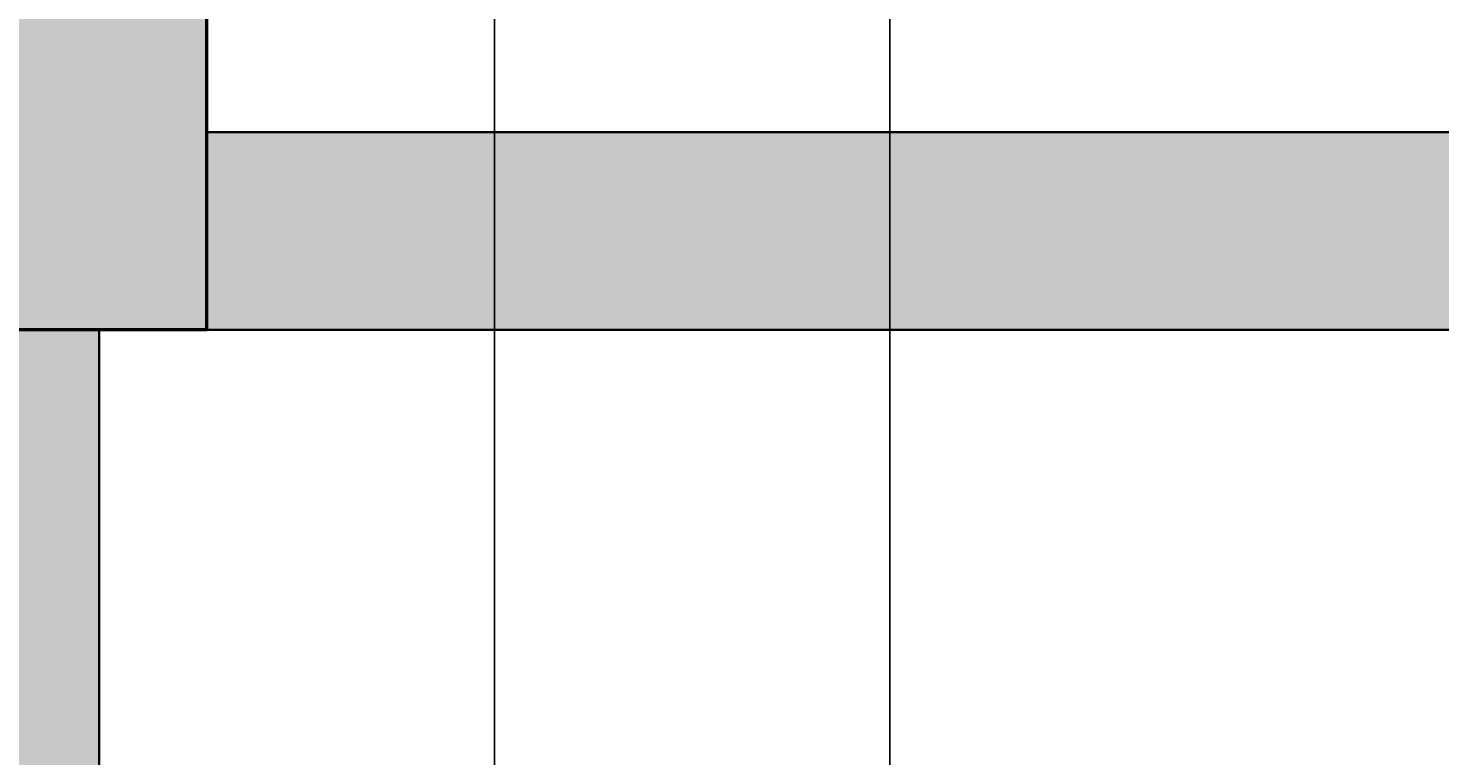
# Model space of a CAD drawing. Units: inches. Extents: x 1998 to 2588, y 1139 to 1977.
# Tile 61 of 134: x 2095 to 2127, y 1746 to 1762. Entities that reach past the tile are written whole.
import ezdxf

# ---------------------------------------------------------------- set-up
doc = ezdxf.new("R2010")
doc.units = ezdxf.units.IN
for name, color, linetype, lineweight in [('A-ANNO-DIMS', 2, 'Continuous', 18), ('A-COLS-PATT', 250, 'Continuous', 13), ('A-WALL-PATT', 252, 'Continuous', 13), ('COLUMN', 10, 'Continuous', 50), ('WALL', 200, 'Continuous', 35)]:
    doc.layers.add(name, color=color, linetype=linetype, lineweight=lineweight)
doc.styles.get("Standard").update_dxf_attribs({"font": 'arial.ttf'})
doc.dimstyles.get("Standard").update_dxf_attribs({"dimtxt": 0.18, "dimasz": 0.18, "dimexe": 0.18, "dimexo": 0.0625, "dimgap": 0.09, "dimtad": 0, "dimtih": 1, "dimtoh": 1, "dimdec": 4, "dimzin": 0, "dimdsep": 46, "dimtxsty": 'Standard', "dimcen": 0.09, "dimadec": 0, "dimazin": 0, "dimtfac": 1, "dimtdec": 4, "dimtofl": 0, "dimtmove": 0, "dimatfit": 3, "dimfxl": 1, "dimtolj": 1, "dimtzin": 0, "dimarcsym": 0})

# ---------------------------------------------------------------- blocks, each defined once
blk = doc.blocks.new('*D40')
at = {"layer": 'A-ANNO-DIMS', "color": 0, "lineweight": -2, "transparency": 16777216}
for p, q in [((2105.973, 1628.541), (2105.973, 1977.362)), ((2114.973, 1628.804), (2114.973, 1977.362)), ((2106.153, 1977.182), (2110.324, 1977.182)), ((2114.793, 1977.182), (2110.622, 1977.182))]:
    blk.add_line(p, q, dxfattribs=at)
at = {"layer": 'A-ANNO-DIMS', "color": 0, "transparency": 16777216}
for points in [[(2106.153, 1977.212), (2106.153, 1977.152), (2105.973, 1977.182)], [(2114.793, 1977.212), (2114.793, 1977.152), (2114.973, 1977.182)]]:
    blk.add_solid(points, dxfattribs=at)
at = {"layer": 'Defpoints', "color": 0, "transparency": 16777216}
for p in [(2114.973, 1977.182), (2114.973, 1628.742), (2105.973, 1628.478)]:
    blk.add_point(p, dxfattribs=at)
at = {"layer": 'A-ANNO-DIMS', "color": 0, "transparency": 16777216, "insert": (2110.473, 1977.182), "char_height": 0.18, "attachment_point": 5}
blk.add_mtext('\\A1;9', dxfattribs=at)

msp = doc.modelspace()

# ---------------------------------------------------------------- hatches: boundary and pattern name
at = {"layer": 'A-COLS-PATT'}
h = msp.add_hatch(color=256, dxfattribs=at)
h.dxf.hatch_style = 1
h.paths.add_polyline_path([(2099.4125, 1888.7324), (2087.9729, 1888.7324), (2087.9729, 1868.3278), (2099.4125, 1868.3278)])
h.paths.add_polyline_path([(2234.4125, 1888.7324), (2222.9729, 1888.7324), (2222.9729, 1868.3278), (2234.4125, 1868.3278)])
h.paths.add_polyline_path([(2341.4729, 1886.637), (2330.0332, 1886.637), (2330.0332, 1866.2324), (2341.4729, 1866.2324)])
h.paths.add_polyline_path([(2507.8006, 1882.7324), (2487.396, 1882.7324), (2487.396, 1871.2927), (2507.8006, 1871.2927)])
h.paths.add_polyline_path([(2510.9729, 1766.672), (2490.5682, 1766.672), (2490.5682, 1755.2324), (2510.9729, 1755.2324)])
h.paths.add_polyline_path([(2345.9729, 1759.7324), (2334.5332, 1759.7324), (2334.5332, 1739.3278), (2345.9729, 1739.3278)])
h.paths.add_polyline_path([(2234.4125, 1774.3318), (2222.9729, 1774.3318), (2222.9729, 1753.9272), (2234.4125, 1753.9272)])
h.paths.add_polyline_path([(2099.4125, 1775.637), (2087.9729, 1775.637), (2087.9729, 1755.2324), (2099.4125, 1755.2324)])
h.paths.add_polyline_path([(2098.0956, 1593.7241), (2077.691, 1593.7241), (2077.691, 1582.2845), (2098.0956, 1582.2845)])
h.paths.add_polyline_path([(2227.4729, 1604.637), (2216.0332, 1604.637), (2216.0332, 1584.2324), (2227.4729, 1584.2324)])
h.paths.add_polyline_path([(2345.9729, 1647.5211), (2334.5332, 1647.5211), (2334.5332, 1627.1165), (2345.9729, 1627.1165)])
h.paths.add_polyline_path([(2522.3775, 1641.2324), (2501.9729, 1641.2324), (2501.9729, 1629.7927), (2522.3775, 1629.7927)])
h.paths.add_polyline_path([(2522.3775, 1480.7324), (2501.9729, 1480.7324), (2501.9729, 1469.2927), (2522.3775, 1469.2927)])
h.paths.add_polyline_path([(2345.9729, 1488.5616), (2334.5332, 1488.5616), (2334.5332, 1468.1569), (2345.9729, 1468.1569)])
h.paths.add_polyline_path([(2234.4125, 1486.137), (2227.4729, 1486.137), (2227.4729, 1465.7324), (2234.4125, 1465.7324)])
h.paths.add_polyline_path([(2227.4729, 1486.137), (2222.9729, 1486.137), (2222.9729, 1465.7324), (2227.4729, 1465.7324)])
h.paths.add_polyline_path([(2108.3775, 1470.2324), (2087.9729, 1470.2324), (2087.9729, 1458.7927), (2108.3775, 1458.7927)])
h.paths.add_polyline_path([(2096.9729, 1365.5012), (2087.9729, 1365.5012), (2087.9729, 1345.0966), (2096.9729, 1345.0966)])
h.paths.add_polyline_path([(2087.9729, 1365.5012), (2085.5332, 1365.5012), (2085.5332, 1345.0966), (2087.9729, 1345.0966)])
h.paths.add_polyline_path([(2234.4125, 1285.137), (2222.9729, 1285.137), (2222.9729, 1264.7324), (2234.4125, 1264.7324)])
h.paths.add_polyline_path([(2345.9729, 1285.137), (2334.5332, 1285.137), (2334.5332, 1264.7324), (2345.9729, 1264.7324)])
h.paths.add_polyline_path([(2503.1458, 1240.172), (2482.7412, 1240.172), (2482.7412, 1228.7324), (2503.1458, 1228.7324)])
h.paths.add_polyline_path([(2510.9729, 1369.172), (2490.5682, 1369.172), (2490.5682, 1357.7324), (2510.9729, 1357.7324)])
at = {"layer": 'A-WALL-PATT'}
h = msp.add_hatch(color=256, dxfattribs=at)
h.dxf.hatch_style = 1
h.paths.add_polyline_path([(2222.9729, 1888.7324), (2099.4125, 1888.7324), (2099.4125, 1879.7324), (2222.9729, 1879.7324)])
h.paths.add_polyline_path([(2096.9729, 1868.3278), (2087.9729, 1868.3278), (2087.9729, 1775.637), (2096.9729, 1775.637)])
h.paths.add_polyline_path([(2227.4729, 1868.3278), (2222.9729, 1868.3278), (2222.9729, 1774.3318), (2227.4729, 1774.3318)])
h.paths.add_polyline_path([(2188.3019, 1759.7324), (2138.6074, 1759.7324), (2099.4125, 1759.7324), (2099.4125, 1755.2324), (2176.9729, 1755.2324), (2188.3019, 1755.2324)])
h.paths.add_polyline_path([(2087.9729, 1759.7324), (2059.4729, 1759.7324), (2059.4729, 1702.7324), (2087.9729, 1702.7324), (2087.9729, 1707.2324), (2063.9729, 1707.2324), (2063.9729, 1755.2324), (2087.9729, 1755.2324)])
h.paths.add_polyline_path([(2096.9729, 1755.2324), (2087.9729, 1755.2324), (2087.9729, 1707.2324), (2096.9729, 1707.2324)])
h.paths.add_polyline_path([(2187.0461, 1707.2324), (2105.9729, 1707.2324), (2096.9729, 1707.2324), (2087.9729, 1707.2324), (2087.9729, 1702.7324), (2105.9729, 1702.7324), (2114.9729, 1702.7324), (2187.0461, 1702.7324)])
h.paths.add_polyline_path([(2181.4729, 1719.2028), (2176.9729, 1719.2028), (2176.9729, 1707.2324), (2181.4729, 1707.2324)])
h.paths.add_polyline_path([(2216.0332, 1588.7324), (2114.9729, 1588.7324), (2105.9729, 1588.7324), (2105.9729, 1584.2324), (2216.0332, 1584.2324)])
h.paths.add_polyline_path([(2077.691, 1588.7324), (2061.4729, 1588.7324), (2061.4729, 1584.2324), (2077.691, 1584.2324)])
h.paths.add_polyline_path([(2105.9729, 1588.7324), (2098.0956, 1588.7324), (2098.0956, 1584.2324), (2105.9729, 1584.2324)])
h.paths.add_polyline_path([(2114.9729, 1596.2642), (2110.1012, 1596.2642), (2105.9729, 1596.2642), (2105.9729, 1588.7324), (2114.9729, 1588.7324)])
h.paths.add_polyline_path([(2114.9729, 1584.2324), (2105.9729, 1584.2324), (2105.9729, 1580.249), (2110.1012, 1580.249), (2114.9729, 1580.249)])
h.paths.add_polyline_path([(2114.9729, 1547.7716), (2110.1012, 1547.7716, -0.0318759), (2105.9729, 1548.035), (2105.9729, 1470.2324), (2108.3775, 1470.2324), (2108.3775, 1465.7324), (2186.2943, 1465.7324), (2186.2943, 1470.2324), (2114.9729, 1470.2324)])
h.paths.add_polyline_path([(2227.4729, 1584.2324), (2222.9729, 1584.2324), (2222.9729, 1486.137), (2227.4729, 1486.137)])
h.paths.add_polyline_path([(2295.4138, 1593.2324), (2227.4729, 1593.2324), (2227.4729, 1588.7324), (2295.4138, 1588.7324), (2295.4138, 1591.8729)])
h.paths.add_polyline_path([(2345.9729, 1627.1165), (2341.4729, 1627.1165), (2341.4729, 1593.2324), (2337.2869, 1593.2324), (2337.2869, 1591.8729), (2337.2869, 1588.7324), (2345.9729, 1588.7324)])
h.paths.add_polyline_path([(2291.9729, 1588.7324), (2287.4729, 1588.7324), (2287.4729, 1522.7324), (2291.9729, 1522.7324)])
h.paths.add_polyline_path([(2291.9729, 1522.7324), (2287.4729, 1522.7324), (2227.4729, 1522.7324), (2227.4729, 1518.2324), (2291.9729, 1518.2324)])
h.paths.add_polyline_path([(2295.7347, 1519.5919), (2295.7347, 1522.7324), (2291.9729, 1522.7324), (2291.9729, 1518.2324), (2295.7347, 1518.2324)])
h.paths.add_polyline_path([(2345.9729, 1522.7324), (2337.6078, 1522.7324), (2337.6078, 1519.5919), (2337.6078, 1518.2324), (2341.4729, 1518.2324), (2341.4729, 1488.5616), (2345.9729, 1488.5616)])
h.paths.add_polyline_path([(2345.9729, 1468.1569), (2341.4729, 1468.1569), (2341.4729, 1374.2324), (2227.4729, 1374.2324), (2227.4729, 1369.7324), (2345.9729, 1369.7324)])
h.paths.add_polyline_path([(2345.9729, 1369.7324), (2341.4729, 1369.7324), (2341.4729, 1362.2324), (2345.9729, 1362.2324)])
h.paths.add_polyline_path([(2345.9729, 1317.7324), (2345.9729, 1322.2324), (2341.4729, 1322.2324), (2341.4729, 1285.137), (2345.9729, 1285.137)], flags=17)
h.paths.add_polyline_path([(2356.2096, 1322.2324), (2345.9729, 1322.2324), (2345.9729, 1317.7324), (2356.2096, 1317.7324), (2356.2096, 1319.3088)], flags=17)
h.paths.add_polyline_path([(2393.9729, 1322.2324), (2375.6999, 1322.2324), (2375.6999, 1319.3088, -0.0202458), (2375.636, 1317.7324), (2393.9729, 1317.7324)], flags=17)
h.paths.add_polyline_path([(2398.4729, 1322.2324), (2393.9729, 1322.2324), (2393.9729, 1317.7324), (2393.9729, 1237.7324), (2345.9729, 1237.7324), (2345.9729, 1264.7324), (2341.4729, 1264.7324), (2341.4729, 1228.7324), (2393.9729, 1228.7324), (2482.7412, 1228.7324), (2482.7412, 1237.7324), (2398.4729, 1237.7324), (2398.4729, 1297.1029)])
h.paths.add_polyline_path([(2398.4729, 1362.2324), (2393.9729, 1362.2324), (2393.9729, 1357.7324), (2398.4729, 1357.7324)])
h.paths.add_polyline_path([(2345.9729, 1329.7549), (2341.4729, 1329.7549), (2341.4729, 1322.2324), (2345.9729, 1322.2324)])

# ---------------------------------------------------------------- linework, layer by layer
at = {"layer": 'COLUMN'}
msp.add_lwpolyline([(2087.9729, 1775.637), (2099.4125, 1775.637), (2099.4125, 1755.2324), (2087.9729, 1755.2324)], close=True, dxfattribs=at)
at = {"layer": 'WALL'}
for p, q in [((2099.4125, 1759.7324), (2138.6074, 1759.7324)), ((2087.9729, 1755.2324), (2138.6074, 1755.2324)), ((2096.9729, 1755.2324), (2096.9729, 1707.2324)), ((2096.9729, 1755.2324), (2176.9729, 1755.2324))]:
    msp.add_line(p, q, dxfattribs=at)

# ---------------------------------------------------------------- dimensions: what is measured, and where the dimension line sits
at = {"layer": 'A-ANNO-DIMS'}
dim = msp.add_linear_dim(base=(2114.9729, 1977.1824), p1=(2105.9729, 1628.4781), p2=(2114.9729, 1628.7416), dimstyle='Standard', override={"dimdec": 0, "dimlfac": 1, "dimrnd": 0, "dimzin": 0, "dimdsep": 46, "dimlunit": 2}, dxfattribs=at)
dim.commit()
dim.dimension.update_dxf_attribs({"geometry": '*D40', "text_midpoint": (2110.4729, 1977.1824)})

doc.saveas('drawing.dxf')
